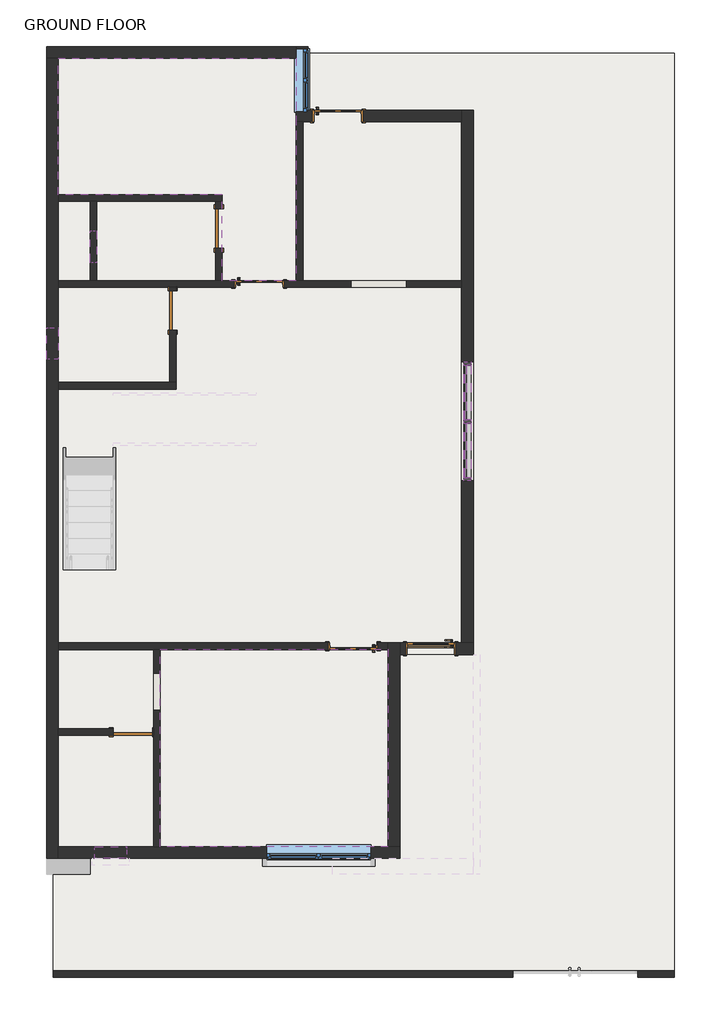
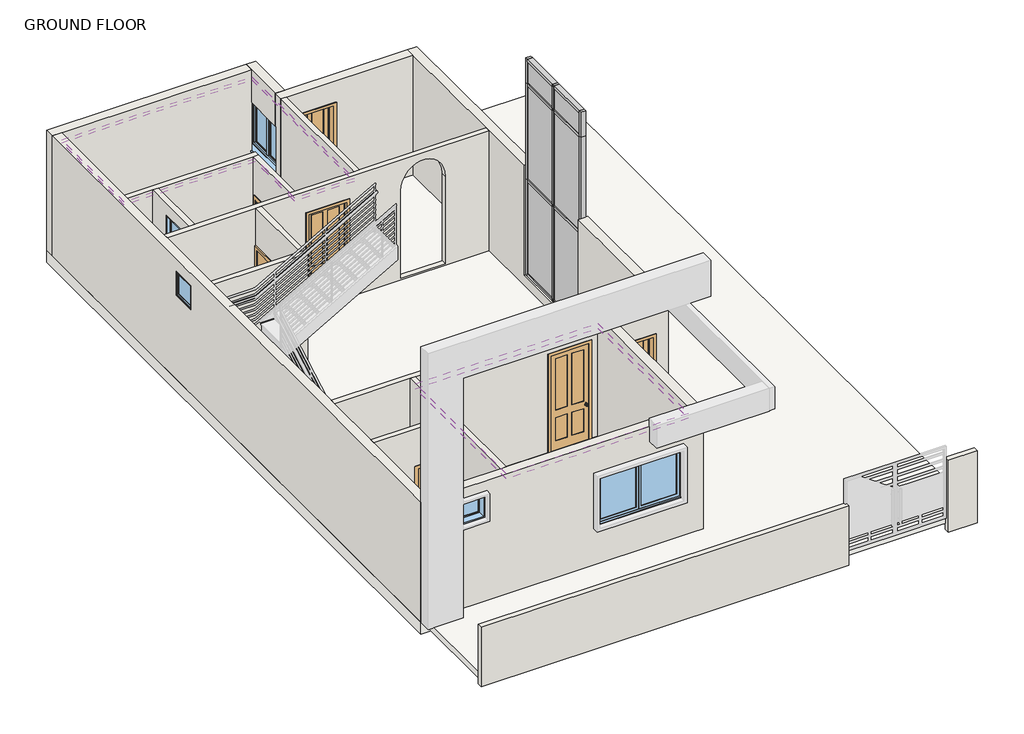
# One storey, part 1 of 3: 20 walls, 17 members, 7 doors, 6 plates, 5 windows, 4 coverings, 3 slabs.
"""IFC4 building model written with IfcOpenShell, lengths in millimetres."""

from ifc_helpers import new_model, si_unit, point, frame, origin, origin_with_axes, place, context, project, spatial, polyline, ellipse_curve, trimmed, outline, extrude, faceted_brep, transform, mapped, element, save
from ifc_brep_helpers import plane_surface, extruded_surface, advanced_brep
from components import door_16625766, door_72f69035, door_4f3f9908, door_1fe7f57d, member_78934672, member_697f972d, member_f0fea5a5, member_ee409385, member_057e2f1d, member_06d1cbbd, system_panel_glazed_cc935e45, system_panel_glazed_66ef8e2c, system_panel_glazed_3447b65c, window_80340324, window_d757e824, w2_window_4_x_4_9dec5fc7, w2_window_6_x_4_7b90d420

model = new_model("IFC4")

# Units and contexts
model_context = context("Model", 3, world=origin())
ifc_project = project(units=[si_unit("LENGTHUNIT", "METRE", prefix="MILLI")], contexts=[model_context])

# Site, building, storey
site = spatial("IfcSite", under=ifc_project)
building = spatial("IfcBuilding", under=site)
storey = spatial("IfcBuildingStorey", under=building, Name="GROUND FLOOR", Elevation=304.8)

# Coverings
placement = place(None, origin())
element("IfcCovering", 1, at=placement, inside=storey, context=model_context, shape_type="SweptSolid", body=[
    extrude(outline(polyline([(-7080.273248, 8978.3133697), (-7080.273248, 11594.5133697), (-2508.273248, 11594.5133697), (-2508.273248, 7327.3133697), (-3930.673248, 7327.3133697), (-3930.673248, 8978.3133697), (-7080.273248, 8978.3133697)]), holes=[polyline([(-6775.473248, 11289.7133697), (-6775.473248, 9283.1133697), (-3625.873248, 9283.1133697), (-3625.873248, 7632.1133697), (-2813.073248, 7632.1133697), (-2813.073248, 11289.7133697), (-6775.473248, 11289.7133697)])]), frame((0.0, 0.0, 3098.8), z_axis=(0.0, 0.0, 1.0), x_axis=(1.0, 0.0, 0.0)), (0.0, 0.0, 1.0), 107.95),
    extrude(outline(polyline([(-3422.673248, 10680.1133697), (-3422.673248, 9892.7133697), (-6165.873248, 9892.7133697), (-6165.873248, 10680.1133697), (-3422.673248, 10680.1133697)])), frame((0.0, 0.0, 3098.8), z_axis=(0.0, 0.0, 1.0), x_axis=(1.0, 0.0, 0.0)), (0.0, 0.0, 1.0), 107.95),
])
element("IfcCovering", 2, ObjectType="METAL STUD WHITE CEILING", at=placement, inside=storey, context=model_context, shape_type="SweptSolid", body=[
    extrude(outline(polyline([(-742.973248, 240.7133697), (-742.973248, -3543.8866303), (-5124.473248, -3543.8866303), (-5124.473248, 240.7133697), (-742.973248, 240.7133697)])), frame((0.0, 0.0, 3175.0), z_axis=(0.0, 0.0, 1.0), x_axis=(1.0, 0.0, 0.0)), (0.0, 0.0, 1.0), 107.95),
])
element("IfcCovering", 3, ObjectType="METAL STUD WHITE CEILING", at=placement, inside=storey, context=model_context, shape_type="SweptSolid", body=[
    extrude(outline(polyline([(-742.973248, 240.7133697), (-742.973248, -3543.8866303), (-5124.473248, -3543.8866303), (-5124.473248, 240.7133697), (-742.973248, 240.7133697)]), holes=[polyline([(-1047.773248, -64.0866303), (-4819.673248, -64.0866303), (-4819.673248, -3239.0866303), (-1047.773248, -3239.0866303), (-1047.773248, -64.0866303)])]), frame((0.0, 0.0, 3048.0), z_axis=(0.0, 0.0, 1.0), x_axis=(1.0, 0.0, 0.0)), (0.0, 0.0, 1.0), 107.95),
])
element("IfcCovering", 4, ObjectType="METAL STUD WHITE CEILING", at=placement, inside=storey, context=model_context, shape_type="SweptSolid", body=[
    extrude(outline(polyline([(-3930.673248, 8978.3133697), (-7080.273248, 8978.3133697), (-7080.273248, 11594.5133697), (-2508.273248, 11594.5133697), (-2508.273248, 10489.6133697), (-2508.273248, 7327.3133697), (-3930.673248, 7327.3133697), (-3930.673248, 8978.3133697)])), frame((0.0, 0.0, 3175.0), z_axis=(0.0, 0.0, 1.0), x_axis=(1.0, 0.0, 0.0)), (0.0, 0.0, 1.0), 107.95),
])

# Doors
door_shape = door_16625766(model_context)
element("IfcDoor", 5, ObjectType="36\" x 84\"", at=placement, inside=storey, context=model_context, shape_type="MappedRepresentation", body=[
    mapped(door_shape, transform((76.176752, 256.5883697, 304.8), x_axis=(1.0, 0.0, 0.0), y_axis=(0.0, 1.0, 0.0), z_axis=(0.0, 0.0, 1.0))),
])
door_2_shape = door_72f69035(model_context)
element("IfcDoor", 6, ObjectType="Door-Interior-Single-4_Panel-Wood : 36\" x 96\"", at=placement, inside=storey, context=model_context, shape_type="MappedRepresentation", body=[
    mapped(door_2_shape, transform((-1416.073248, 301.0383697, 304.8), x_axis=(-1.0, 0.0, 0.0), y_axis=(0.0, -1.0, 0.0), z_axis=(0.0, 0.0, 1.0))),
])
element("IfcDoor", 7, ObjectType="Door-Interior-Single-4_Panel-Wood : 36\" x 96\"", at=placement, inside=storey, context=model_context, shape_type="MappedRepresentation", body=[
    mapped(door_2_shape, transform((-3219.473248, 7266.9883697, 304.8), x_axis=(1.0, 0.0, 0.0), y_axis=(0.0, 1.0, 0.0), z_axis=(0.0, 0.0, 1.0))),
])
door_3_shape = door_4f3f9908(model_context)
element("IfcDoor", 8, ObjectType="Door-Interior-Single-4_Panel-Wood : 36\" x 96\"", at=placement, inside=storey, context=model_context, shape_type="MappedRepresentation", body=[
    mapped(door_3_shape, transform((-1708.173248, 10492.7883697, 304.8), x_axis=(1.0, 0.0, 0.0), y_axis=(0.0, 1.0, 0.0), z_axis=(0.0, 0.0, 1.0))),
])
door_4_shape = door_1fe7f57d(model_context)
element("IfcDoor", 9, ObjectType="Single-Flush : 30\" x 80\"", at=placement, inside=storey, context=model_context, shape_type="MappedRepresentation", body=[
    mapped(door_4_shape, transform((-4883.173248, 6755.8133697, 304.8), x_axis=(0.0, 1.0, 0.0), y_axis=(-1.0, 0.0, 0.0), z_axis=(0.0, 0.0, 1.0))),
])
element("IfcDoor", 10, ObjectType="Single-Flush : 30\" x 80\"", at=placement, inside=storey, context=model_context, shape_type="MappedRepresentation", body=[
    mapped(door_4_shape, transform((-3994.173248, 8330.6133697, 304.8), x_axis=(0.0, 1.0, 0.0), y_axis=(-1.0, 0.0, 0.0), z_axis=(0.0, 0.0, 1.0))),
])
element("IfcDoor", 11, ObjectType="Single-Flush : 30\" x 80\"", at=placement, inside=storey, context=model_context, shape_type="MappedRepresentation", body=[
    mapped(door_4_shape, transform((-5645.173248, -1346.7866303, 304.8), x_axis=(-1.0, 0.0, 0.0), y_axis=(0.0, -1.0, 0.0), z_axis=(0.0, 0.0, 1.0))),
])

# Members
member_shape = member_78934672(model_context)
element("IfcMember", 12, ObjectType="Rectangular Mullion : 2.5\" x 5\" rectangular", at=placement, inside=storey, context=model_context, shape_type="MappedRepresentation", body=[
    mapped(member_shape, transform((781.026752, 5701.7133697, 6059.5090117), x_axis=(0.0, 0.0, 1.0), y_axis=(1.0, 0.0, 0.0), z_axis=(0.0, 1.0, 0.0))),
])
element("IfcMember", 13, ObjectType="Rectangular Mullion : 2.5\" x 5\" rectangular", at=placement, inside=storey, context=model_context, shape_type="MappedRepresentation", body=[
    mapped(member_shape, transform((781.026752, 4590.4633697, 6059.5090117), x_axis=(0.0, 0.0, 1.0), y_axis=(1.0, 0.0, 0.0), z_axis=(0.0, 1.0, 0.0))),
])
element("IfcMember", 14, ObjectType="Rectangular Mullion : 2.5\" x 5\" rectangular", at=placement, inside=storey, context=model_context, shape_type="MappedRepresentation", body=[
    mapped(member_shape, transform((781.026752, 3542.7133697, 546.4883491), x_axis=(0.0, 0.0, -1.0), y_axis=(1.0, 0.0, 0.0), z_axis=(0.0, -1.0, 0.0))),
])
element("IfcMember", 15, ObjectType="Rectangular Mullion : 2.5\" x 5\" rectangular", at=placement, inside=storey, context=model_context, shape_type="MappedRepresentation", body=[
    mapped(member_shape, transform((781.026752, 4653.9633697, 546.4883491), x_axis=(0.0, 0.0, -1.0), y_axis=(1.0, 0.0, 0.0), z_axis=(0.0, -1.0, 0.0))),
])
member_2_shape = member_697f972d(model_context)
element("IfcMember", 16, ObjectType="Rectangular Mullion : 2.5\" x 5\" rectangular", at=placement, inside=storey, context=model_context, shape_type="MappedRepresentation", body=[
    mapped(member_2_shape, transform((781.026752, 4590.4633697, 2984.8883491), x_axis=(0.0, 0.0, 1.0), y_axis=(1.0, 0.0, 0.0), z_axis=(0.0, 1.0, 0.0))),
])
element("IfcMember", 17, ObjectType="Rectangular Mullion : 2.5\" x 5\" rectangular", at=placement, inside=storey, context=model_context, shape_type="MappedRepresentation", body=[
    mapped(member_2_shape, transform((781.026752, 5701.7133697, 2984.8883491), x_axis=(0.0, 0.0, 1.0), y_axis=(1.0, 0.0, 0.0), z_axis=(0.0, 1.0, 0.0))),
])
element("IfcMember", 18, ObjectType="Rectangular Mullion : 2.5\" x 5\" rectangular", at=placement, inside=storey, context=model_context, shape_type="MappedRepresentation", body=[
    mapped(member_2_shape, transform((781.026752, 4590.4633697, 5423.2883491), x_axis=(0.0, 0.0, 1.0), y_axis=(1.0, 0.0, 0.0), z_axis=(0.0, 1.0, 0.0))),
])
element("IfcMember", 19, ObjectType="Rectangular Mullion : 2.5\" x 5\" rectangular", at=placement, inside=storey, context=model_context, shape_type="MappedRepresentation", body=[
    mapped(member_2_shape, transform((781.026752, 5701.7133697, 5423.2883491), x_axis=(0.0, 0.0, 1.0), y_axis=(1.0, 0.0, 0.0), z_axis=(0.0, 1.0, 0.0))),
])
member_3_shape = member_f0fea5a5(model_context)
element("IfcMember", 20, ObjectType="Rectangular Mullion : 2.5\" x 5\" rectangular", at=placement, inside=storey, context=model_context, shape_type="MappedRepresentation", body=[
    mapped(member_3_shape, transform((781.026752, 4622.2133697, 546.4883491), x_axis=(0.0, 1.0, 0.0), y_axis=(1.0, 0.0, 0.0), z_axis=(0.0, 0.0, -1.0))),
])
member_4_shape = member_ee409385(model_context)
element("IfcMember", 21, ObjectType="Rectangular Mullion : 2.5\" x 5\" rectangular", at=placement, inside=storey, context=model_context, shape_type="MappedRepresentation", body=[
    mapped(member_4_shape, transform((781.026752, 5765.2133697, 546.4883491), x_axis=(0.0, 1.0, 0.0), y_axis=(1.0, 0.0, 0.0), z_axis=(0.0, 0.0, -1.0))),
])
element("IfcMember", 22, ObjectType="Rectangular Mullion : 2.5\" x 5\" rectangular", at=placement, inside=storey, context=model_context, shape_type="MappedRepresentation", body=[
    mapped(member_4_shape, transform((781.026752, 3479.2133697, 2984.8883491), x_axis=(0.0, -1.0, 0.0), y_axis=(1.0, 0.0, 0.0), z_axis=(0.0, 0.0, 1.0))),
])
element("IfcMember", 23, ObjectType="Rectangular Mullion : 2.5\" x 5\" rectangular", at=placement, inside=storey, context=model_context, shape_type="MappedRepresentation", body=[
    mapped(member_3_shape, transform((781.026752, 4622.2133697, 2984.8883491), x_axis=(0.0, 1.0, 0.0), y_axis=(1.0, 0.0, 0.0), z_axis=(0.0, 0.0, -1.0))),
])
element("IfcMember", 24, ObjectType="Rectangular Mullion : 2.5\" x 5\" rectangular", at=placement, inside=storey, context=model_context, shape_type="MappedRepresentation", body=[
    mapped(member_4_shape, transform((781.026752, 5765.2133697, 2984.8883491), x_axis=(0.0, 1.0, 0.0), y_axis=(1.0, 0.0, 0.0), z_axis=(0.0, 0.0, -1.0))),
])
element("IfcMember", 25, ObjectType="Rectangular Mullion : 2.5\" x 5\" rectangular", at=placement, inside=storey, context=model_context, shape_type="MappedRepresentation", body=[
    mapped(member_4_shape, transform((781.026752, 3479.2133697, 5423.2883491), x_axis=(0.0, -1.0, 0.0), y_axis=(1.0, 0.0, 0.0), z_axis=(0.0, 0.0, 1.0))),
])
member_5_shape = member_057e2f1d(model_context)
element("IfcMember", 26, ObjectType="Rectangular Mullion : 2.5\" x 5\" rectangular", at=placement, inside=storey, context=model_context, shape_type="MappedRepresentation", body=[
    mapped(member_5_shape, transform((781.026752, 4622.2133697, 5423.2883491), x_axis=(0.0, 1.0, 0.0), y_axis=(1.0, 0.0, 0.0), z_axis=(0.0, 0.0, -1.0))),
])
member_6_shape = member_06d1cbbd(model_context)
element("IfcMember", 27, ObjectType="Rectangular Mullion : 2.5\" x 5\" rectangular", at=placement, inside=storey, context=model_context, shape_type="MappedRepresentation", body=[
    mapped(member_6_shape, transform((781.026752, 3479.2133697, 6059.5090117), x_axis=(0.0, -1.0, 0.0), y_axis=(1.0, 0.0, 0.0), z_axis=(0.0, 0.0, 1.0))),
])
element("IfcMember", 28, ObjectType="Rectangular Mullion : 2.5\" x 5\" rectangular", at=placement, inside=storey, context=model_context, shape_type="MappedRepresentation", body=[
    mapped(member_6_shape, transform((781.026752, 5765.2133697, 5423.2883491), x_axis=(0.0, 1.0, 0.0), y_axis=(1.0, 0.0, 0.0), z_axis=(0.0, 0.0, -1.0))),
])

# Plates
system_panel_glazed_shape = system_panel_glazed_cc935e45(model_context)
element("IfcPlate", 29, ObjectType="System Panel : Glazed", at=placement, inside=storey, context=model_context, shape_type="MappedRepresentation", body=[
    mapped(system_panel_glazed_shape, transform((781.026752, 4066.5883697, 609.9883491), x_axis=(0.0, 1.0, 0.0), y_axis=(-1.0, 0.0, 0.0), z_axis=(0.0, 0.0, 1.0))),
])
element("IfcPlate", 30, ObjectType="System Panel : Glazed", at=placement, inside=storey, context=model_context, shape_type="MappedRepresentation", body=[
    mapped(system_panel_glazed_shape, transform((781.026752, 5177.8383697, 609.9883491), x_axis=(0.0, 1.0, 0.0), y_axis=(-1.0, 0.0, 0.0), z_axis=(0.0, 0.0, 1.0))),
])
system_panel_glazed_2_shape = system_panel_glazed_66ef8e2c(model_context)
element("IfcPlate", 31, ObjectType="System Panel : Glazed", at=placement, inside=storey, context=model_context, shape_type="MappedRepresentation", body=[
    mapped(system_panel_glazed_2_shape, transform((781.026752, 4066.5883697, 3016.6383491), x_axis=(0.0, 1.0, 0.0), y_axis=(-1.0, 0.0, 0.0), z_axis=(0.0, 0.0, 1.0))),
])
element("IfcPlate", 32, ObjectType="System Panel : Glazed", at=placement, inside=storey, context=model_context, shape_type="MappedRepresentation", body=[
    mapped(system_panel_glazed_2_shape, transform((781.026752, 5177.8383697, 3016.6383491), x_axis=(0.0, 1.0, 0.0), y_axis=(-1.0, 0.0, 0.0), z_axis=(0.0, 0.0, 1.0))),
])
system_panel_glazed_3_shape = system_panel_glazed_3447b65c(model_context)
element("IfcPlate", 33, ObjectType="System Panel : Glazed", at=placement, inside=storey, context=model_context, shape_type="MappedRepresentation", body=[
    mapped(system_panel_glazed_3_shape, transform((781.026752, 4066.5883697, 5455.0383491), x_axis=(0.0, 1.0, 0.0), y_axis=(-1.0, 0.0, 0.0), z_axis=(0.0, 0.0, 1.0))),
])
element("IfcPlate", 34, ObjectType="System Panel : Glazed", at=placement, inside=storey, context=model_context, shape_type="MappedRepresentation", body=[
    mapped(system_panel_glazed_3_shape, transform((781.026752, 5177.8383697, 5455.0383491), x_axis=(0.0, 1.0, 0.0), y_axis=(-1.0, 0.0, 0.0), z_axis=(0.0, 0.0, 1.0))),
])

# Slabs
element("IfcSlab", 35, at=placement, inside=storey, context=model_context, shape_type="SweptSolid", body=[
    extrude(outline(polyline([(-5251.473248, -3543.8866303), (-7080.273248, -3543.8866303), (-7080.273248, -1410.2866303), (-5251.473248, -1410.2866303), (-5251.473248, -3543.8866303)])), origin_with_axes(), (0.0, 0.0, 1.0), 304.8),
    extrude(outline(polyline([(-4946.673248, 7200.3133697), (-4946.673248, 5371.5133697), (-7080.273248, 5371.5133697), (-7080.273248, 7200.3133697), (-4946.673248, 7200.3133697)])), origin_with_axes(), (0.0, 0.0, 1.0), 304.8),
    extrude(outline(polyline([(-4057.673248, 8851.3133697), (-4057.673248, 7327.3133697), (-6343.673248, 7327.3133697), (-6343.673248, 8851.3133697), (-4057.673248, 8851.3133697)])), origin_with_axes(), (0.0, 0.0, 1.0), 304.8),
])
element("IfcSlab", 36, at=placement, inside=storey, context=model_context, shape_type="SweptSolid", body=[
    extrude(outline(polyline([(-514.373248, -3772.4866303), (-514.373248, 139.1133697), (895.326752, 139.1133697), (895.326752, 10603.9133697), (-2279.673248, 10603.9133697), (-2279.673248, 11696.1133697), (4756.126752, 11696.1133697), (4756.126752, -5931.4866303), (-7181.873248, -5931.4866303), (-7181.873248, -3772.4866303), (-514.373248, -3772.4866303)])), frame((0.0, 0.0, 152.4), z_axis=(0.0, 0.0, 1.0), x_axis=(1.0, 0.0, 0.0)), (0.0, 0.0, 1.0), 152.4),
])
element("IfcSlab", 37, ObjectType="MARBLE FLOORING 1'", at=placement, inside=storey, context=model_context, shape_type="SweptSolid", body=[
    extrude(outline(polyline([(-514.373248, -3772.4866303), (-7308.873248, -3772.4866303), (-7308.873248, 11823.1133697), (-2279.673248, 11823.1133697), (-2279.673248, 10603.9133697), (895.326752, 10603.9133697), (895.326752, 139.1133697), (-514.373248, 139.1133697), (-514.373248, -3772.4866303)]), holes=[polyline([(-4057.673248, 8851.3133697), (-6343.673248, 8851.3133697), (-6343.673248, 7327.3133697), (-4057.673248, 7327.3133697), (-4057.673248, 8851.3133697)]), polyline([(-4946.673248, 7200.3133697), (-7080.273248, 7200.3133697), (-7080.273248, 5371.5133697), (-4946.673248, 5371.5133697), (-4946.673248, 7200.3133697)]), polyline([(-5251.473248, -3543.8866303), (-5251.473248, -1410.2866303), (-7080.273248, -1410.2866303), (-7080.273248, -3543.8866303), (-5251.473248, -3543.8866303)])]), origin_with_axes(), (0.0, 0.0, 1.0), 304.8),
])

# Walls
element("IfcWall", 38, ObjectType="INNER WALL 5\"", at=placement, inside=storey, context=model_context, shape_type="AdvancedBrep", body=[
    advanced_brep(
    [(-5124.473248, -3543.8866303, 304.8), (-5124.473248, 240.7133697, 304.8), (-5124.473248, 240.7133697, 3352.8), (-5124.473248, -3543.8866303, 3352.8), (-5124.473248, -211.107669, 445.0989834), (-5124.473248, -921.3329942, 445.0989834), (-5124.473248, -921.3329942, 2667.1596494), (-5124.473248, -211.107669, 2629.9383173), (-5251.473248, -3543.8866303, 304.8), (-5251.473248, -3543.8866303, 3352.8), (-5251.473248, -1410.2866303, 3352.8), (-5251.473248, -1283.2866303, 3352.8), (-5251.473248, 240.7133697, 3352.8), (-5251.473248, 240.7133697, 304.8), (-5251.473248, -1283.2866303, 304.8), (-5251.473248, -1410.2866303, 304.8), (-5251.473248, -211.107669, 445.0989834), (-5251.473248, -211.107669, 2629.9383173), (-5251.473248, -921.3329942, 2667.1596494), (-5251.473248, -921.3329942, 445.0989834)],
    [
        (0, 1),
        (1, 2),
        (2, 3),
        (3, 0),
        (4, 5),
        (5, 6),
        (6, 7, ellipse_curve(frame((-5124.473248, -566.2203316, 2648.5489834), z_axis=(-1.0, 0.0, 0.0), x_axis=(0.0, -0.052335956242941746, -0.998629534754574)), 457.2, 355.6)),
        (7, 4),
        (8, 9),
        (9, 10),
        (10, 11),
        (11, 12),
        (12, 13),
        (13, 14),
        (14, 15),
        (15, 8),
        (16, 17),
        (17, 18, ellipse_curve(frame((-5251.473248, -566.2203316, 2648.5489834), z_axis=(1.0, 0.0, 0.0), x_axis=(0.0, -0.052335956242941746, -0.998629534754574)), 457.2, 355.6)),
        (18, 19),
        (19, 16),
        (3, 9),
        (8, 0),
        (1, 13),
        (12, 2),
        (4, 16),
        (19, 5),
        (18, 6),
        (17, 7),
    ],
    [
        plane_surface(frame((-5124.473248, -3543.8866303, 304.8), z_axis=(1.0, 0.0, 0.0), x_axis=(0.0, 1.0, 0.0))),
        plane_surface(frame((-5251.473248, -3543.8866303, 304.8), z_axis=(-1.0, 0.0, 0.0), x_axis=(0.0, -1.0, 0.0))),
        plane_surface(frame((-7219.973248, -3543.8866303, 304.8), z_axis=(0.0, -1.0, 0.0), x_axis=(-1.0, 0.0, 0.0))),
        plane_surface(frame((-742.973248, 240.7133697, 304.8), z_axis=(0.0, 1.0, 0.0), x_axis=(1.0, 0.0, 0.0))),
        plane_surface(frame((-5124.473248, -3658.1866303, 304.8), z_axis=(0.0, 0.0, -1.0), x_axis=(-1.0, 0.0, 0.0))),
        plane_surface(frame((-5124.473248, 304.2133697, 3352.8), z_axis=(0.0, 0.0, 1.0), x_axis=(-1.0, 0.0, 0.0))),
        plane_surface(frame((-5124.473248, -211.107669, 445.0989834), z_axis=(0.0, 0.0, 1.0), x_axis=(-1.0, 0.0, 0.0))),
        plane_surface(frame((-5124.473248, -921.3329942, 445.0989834), z_axis=(0.0, 1.0, 0.0), x_axis=(-1.0, 0.0, 0.0))),
        extruded_surface(trimmed(ellipse_curve(frame((-5314.973248, -566.2203316, 2648.5489834), z_axis=(-1.0, 0.0, 0.0), x_axis=(0.0, 0.998629534754574, -0.052335956242941746)), 355.6, 457.2), [point((-5314.973248, -921.3329942, 2667.1596494))], [point((-5314.973248, -211.107669, 2629.9383173))], True, "CARTESIAN"), (127.0, 0.0, 0.0), 127.0),
        plane_surface(frame((-5124.473248, -211.107669, 2629.9383173), z_axis=(0.0, -1.0, 0.0), x_axis=(-1.0, 0.0, 0.0))),
    ],
    [
        (0, [[1, 2, 3, 4], [5, 6, 7, 8]]),
        (1, [[9, 10, 11, 12, 13, 14, 15, 16], [17, 18, 19, 20]]),
        (2, [[-4, 21, -9, 22]]),
        (3, [[-2, 23, -13, 24]]),
        (4, [[-1, -22, -16, -15, -14, -23]]),
        (5, [[-3, -24, -12, -11, -10, -21]]),
        (6, [[-5, 25, -20, 26]]),
        (7, [[-6, -26, -19, 27]]),
        (8, [[-7, -27, -18, 28]]),
        (9, [[-8, -28, -17, -25]]),
    ],
),
])
element("IfcWall", 39, ObjectType="INNER WALL 5\"", at=placement, inside=storey, context=model_context, shape_type="SweptSolid", body=[
    extrude(outline(polyline([(304.8, -7080.273248), (304.8, -6026.173248), (2336.8, -6026.173248), (2336.8, -5264.173248), (304.8, -5264.173248), (304.8, -5251.473248), (3352.8, -5251.473248), (3352.8, -7080.273248), (304.8, -7080.273248)])), frame((0.0, -1410.2866303, 0.0), z_axis=(0.0, 1.0, 0.0), x_axis=(0.0, 0.0, 1.0)), (0.0, 0.0, 1.0), 127.0),
])
element("IfcWall", 40, ObjectType="INNER WALL 5\"", at=placement, inside=storey, context=model_context, shape_type="Brep", body=[
    faceted_brep([(-7080.273248, 367.7133697, 3352.8), (-742.973248, 367.7133697, 3352.8), (-742.973248, 367.7133697, 304.8), (-933.473248, 367.7133697, 304.8), (-933.473248, 367.7133697, 2768.6), (-1898.673248, 367.7133697, 2768.6), (-1898.673248, 367.7133697, 304.8), (-7080.273248, 367.7133697, 304.8), (-742.973248, 240.7133697, 3352.8), (-5124.473248, 240.7133697, 3352.8), (-5251.473248, 240.7133697, 3352.8), (-7080.273248, 240.7133697, 3352.8), (-7080.273248, 240.7133697, 304.8), (-5251.473248, 240.7133697, 304.8), (-5124.473248, 240.7133697, 304.8), (-1898.673248, 240.7133697, 304.8), (-1898.673248, 240.7133697, 2768.6), (-933.473248, 240.7133697, 2768.6), (-933.473248, 240.7133697, 304.8), (-742.973248, 240.7133697, 304.8)], [[[0, 1, 2, 3, 4, 5, 6, 7]], [[8, 9, 10, 11, 12, 13, 14, 15, 16, 17, 18, 19]], [[2, 19, 18, 3]], [[12, 7, 6, 15, 14, 13]], [[1, 0, 11, 10, 9, 8]], [[2, 1, 8, 19]], [[0, 7, 12, 11]], [[5, 16, 15, 6]], [[16, 5, 4, 17]], [[17, 4, 3, 18]]]),
])
element("IfcWall", 41, ObjectType="INNER WALL 5\"", at=placement, inside=storey, context=model_context, shape_type="AdvancedBrep", body=[
    advanced_brep(
    [(666.726752, 7200.3133697, 3352.8), (-4819.673248, 7200.3133697, 3352.8), (-4946.673248, 7200.3133697, 3352.8), (-7080.273248, 7200.3133697, 3352.8), (-7080.273248, 7200.3133697, 304.8), (-4946.673248, 7200.3133697, 304.8), (-4819.673248, 7200.3133697, 304.8), (-3702.073248, 7200.3133697, 304.8), (-3702.073248, 7200.3133697, 2768.6), (-2736.873248, 7200.3133697, 2768.6), (-2736.873248, 7200.3133697, 304.8), (666.726752, 7200.3133697, 304.8), (-387.8615631, 7200.3133697, 344.0138877), (-1454.6615631, 7200.3133697, 344.0138877), (-1454.6615631, 7200.3133697, 2318.5977751), (-1454.6615631, 7200.3133697, 2566.5138877), (-387.8615631, 7200.3133697, 2566.5138877), (-7080.273248, 7327.3133697, 3352.8), (-6470.673248, 7327.3133697, 3352.8), (-6343.673248, 7327.3133697, 3352.8), (-4057.673248, 7327.3133697, 3352.8), (-3930.673248, 7327.3133697, 3352.8), (-2508.273248, 7327.3133697, 3352.8), (-2381.273248, 7327.3133697, 3352.8), (666.726752, 7327.3133697, 3352.8), (666.726752, 7327.3133697, 304.8), (-2381.273248, 7327.3133697, 304.8), (-2508.273248, 7327.3133697, 304.8), (-2736.873248, 7327.3133697, 304.8), (-2736.873248, 7327.3133697, 2768.6), (-3702.073248, 7327.3133697, 2768.6), (-3702.073248, 7327.3133697, 304.8), (-3930.673248, 7327.3133697, 304.8), (-4057.673248, 7327.3133697, 304.8), (-6343.673248, 7327.3133697, 304.8), (-6470.673248, 7327.3133697, 304.8), (-7080.273248, 7327.3133697, 304.8), (-1454.6615631, 7327.3133697, 344.0138877), (-387.8615631, 7327.3133697, 344.0138877), (-387.8615631, 7327.3133697, 2566.5138877), (-1454.6615631, 7327.3133697, 2566.5138877), (-1454.6615631, 7327.3133697, 2318.5977751)],
    [
        (0, 1),
        (1, 2),
        (2, 3),
        (3, 4),
        (4, 5),
        (5, 6),
        (6, 7),
        (7, 8),
        (8, 9),
        (9, 10),
        (10, 11),
        (11, 0),
        (12, 13),
        (13, 14),
        (14, 15),
        (15, 16, ellipse_curve(frame((-921.2615631, 7200.3133697, 2566.5138877), z_axis=(0.0, 1.0, 0.0), x_axis=(0.0, 0.0, -1.0)), 609.6, 533.4)),
        (16, 12),
        (17, 18),
        (18, 19),
        (19, 20),
        (20, 21),
        (21, 22),
        (22, 23),
        (23, 24),
        (24, 25),
        (25, 26),
        (26, 27),
        (27, 28),
        (28, 29),
        (29, 30),
        (30, 31),
        (31, 32),
        (32, 33),
        (33, 34),
        (34, 35),
        (35, 36),
        (36, 17),
        (37, 38),
        (38, 39),
        (39, 40, ellipse_curve(frame((-921.2615631, 7327.3133697, 2566.5138877), z_axis=(0.0, -1.0, 0.0), x_axis=(0.0, 0.0, -1.0)), 609.6, 533.4)),
        (40, 41),
        (41, 37),
        (3, 17),
        (36, 4),
        (11, 25),
        (24, 0),
        (31, 7),
        (10, 28),
        (12, 38),
        (37, 13),
        (41, 14),
        (40, 15),
        (39, 16),
        (9, 29),
        (8, 30),
    ],
    [
        plane_surface(frame((-6991.373248, 7200.3133697, 304.8), z_axis=(0.0, -1.0, 0.0), x_axis=(1.0, 0.0, 0.0))),
        plane_surface(frame((-6991.373248, 7327.3133697, 304.8), z_axis=(0.0, 1.0, 0.0), x_axis=(-1.0, 0.0, 0.0))),
        plane_surface(frame((-7080.273248, 8571.9133697, 304.8), z_axis=(-1.0, 0.0, 0.0), x_axis=(0.0, 1.0, 0.0))),
        plane_surface(frame((666.726752, 1256.7133697, 304.8), z_axis=(1.0, 0.0, 0.0), x_axis=(0.0, -1.0, 0.0))),
        plane_surface(frame((-7194.573248, 7200.3133697, 304.8), z_axis=(0.0, 0.0, -1.0), x_axis=(0.0, 1.0, 0.0))),
        plane_surface(frame((781.026752, 7200.3133697, 3352.8), z_axis=(0.0, 0.0, 1.0), x_axis=(0.0, 1.0, 0.0))),
        plane_surface(frame((-387.8615631, 7200.3133697, 344.0138877), z_axis=(0.0, 0.0, 1.0), x_axis=(0.0, 1.0, 0.0))),
        plane_surface(frame((-1454.6615631, 7200.3133697, 344.0138877), z_axis=(1.0, 0.0, 0.0), x_axis=(0.0, 1.0, 0.0))),
        plane_surface(frame((-1454.6615631, 7200.3133697, 2318.5977751), z_axis=(1.0, 0.0, 0.0), x_axis=(0.0, 1.0, 0.0))),
        extruded_surface(trimmed(ellipse_curve(frame((-921.2615631, 7390.8133697, 2566.5138877), z_axis=(0.0, 1.0, 0.0), x_axis=(1.0, 0.0, 0.0)), 533.4, 609.6), [point((-1454.6615631, 7390.8133697, 2566.5138877))], [point((-387.8615631, 7390.8133697, 2566.5138877))], True, "CARTESIAN"), (0.0, -127.0, 0.0), 127.0),
        plane_surface(frame((-387.8615631, 7200.3133697, 2566.5138877), z_axis=(-1.0, 0.0, 0.0), x_axis=(0.0, 1.0, 0.0))),
        plane_surface(frame((-2736.873248, 5676.3133697, 304.8), z_axis=(-1.0, 0.0, 0.0), x_axis=(0.0, 1.0, 0.0))),
        plane_surface(frame((-2736.873248, 5676.3133697, 2768.6), z_axis=(0.0, 0.0, -1.0), x_axis=(0.0, 1.0, 0.0))),
        plane_surface(frame((-3702.073248, 5676.3133697, 2768.6), z_axis=(1.0, 0.0, 0.0), x_axis=(0.0, 1.0, 0.0))),
    ],
    [
        (0, [[1, 2, 3, 4, 5, 6, 7, 8, 9, 10, 11, 12], [13, 14, 15, 16, 17]]),
        (1, [[18, 19, 20, 21, 22, 23, 24, 25, 26, 27, 28, 29, 30, 31, 32, 33, 34, 35, 36, 37], [38, 39, 40, 41, 42]]),
        (2, [[-4, 43, -37, 44]]),
        (3, [[-12, 45, -25, 46]]),
        (4, [[-44, -36, -35, -34, -33, -32, 47, -7, -6, -5]]),
        (4, [[-45, -11, 48, -28, -27, -26]]),
        (5, [[-3, -2, -1, -46, -24, -23, -22, -21, -20, -19, -18, -43]]),
        (6, [[-13, 49, -38, 50]]),
        (7, [[-14, -50, -42, 51]]),
        (8, [[-15, -51, -41, 52]]),
        (9, [[-16, -52, -40, 53]]),
        (10, [[-17, -53, -39, -49]]),
        (11, [[54, -29, -48, -10]]),
        (12, [[-54, -9, 55, -30]]),
        (13, [[-55, -8, -47, -31]]),
    ],
),
])
element("IfcWall", 42, ObjectType="INNER WALL 5\"", at=placement, inside=storey, context=model_context, shape_type="SweptSolid", body=[
    extrude(outline(polyline([(-2508.273248, 7327.3133697), (-2508.273248, 10375.3133697), (-2381.273248, 10375.3133697), (-2381.273248, 7327.3133697), (-2508.273248, 7327.3133697)])), frame((0.0, 0.0, 304.8), z_axis=(0.0, 0.0, 1.0), x_axis=(1.0, 0.0, 0.0)), (0.0, 0.0, 1.0), 3048.0),
])
element("IfcWall", 43, ObjectType="INNER WALL 5\"", at=placement, inside=storey, context=model_context, shape_type="Brep", body=[
    faceted_brep([(-7080.273248, 5244.5133697, 304.8), (-4819.673248, 5244.5133697, 304.8), (-4819.673248, 5244.5133697, 3352.8), (-7080.273248, 5244.5133697, 3352.8), (-7080.273248, 5371.5133697, 304.8), (-7080.273248, 5371.5133697, 3352.8), (-4946.673248, 5371.5133697, 3352.8), (-4819.673248, 5371.5133697, 3352.8), (-4819.673248, 5371.5133697, 304.8), (-4946.673248, 5371.5133697, 304.8)], [[[0, 1, 2, 3]], [[4, 5, 6, 7, 8, 9]], [[1, 0, 4, 9, 8]], [[3, 2, 7, 6, 5]], [[0, 3, 5, 4]], [[2, 1, 8, 7]]]),
])
element("IfcWall", 44, ObjectType="INNER WALL 5\"", at=placement, inside=storey, context=model_context, shape_type="SweptSolid", body=[
    extrude(outline(polyline([(7200.3133697, 304.8), (7136.8133697, 304.8), (7136.8133697, 2336.8), (6374.8133697, 2336.8), (6374.8133697, 304.8), (5371.5133697, 304.8), (5371.5133697, 3352.8), (7200.3133697, 3352.8), (7200.3133697, 304.8)])), frame((-4946.673248, 0.0, 0.0), z_axis=(1.0, 0.0, 0.0), x_axis=(0.0, 1.0, 0.0)), (0.0, 0.0, 1.0), 127.0),
])
element("IfcWall", 45, ObjectType="INNER WALL 5\"", at=placement, inside=storey, context=model_context, shape_type="Brep", body=[
    faceted_brep([(-7080.273248, 8851.3133697, 304.8), (-6470.673248, 8851.3133697, 304.8), (-6343.673248, 8851.3133697, 304.8), (-4057.673248, 8851.3133697, 304.8), (-3930.673248, 8851.3133697, 304.8), (-3930.673248, 8851.3133697, 3352.8), (-4057.673248, 8851.3133697, 3352.8), (-6343.673248, 8851.3133697, 3352.8), (-6470.673248, 8851.3133697, 3352.8), (-7080.273248, 8851.3133697, 3352.8), (-7080.273248, 8978.3133697, 304.8), (-7080.273248, 8978.3133697, 3352.8), (-3930.673248, 8978.3133697, 3352.8), (-3930.673248, 8978.3133697, 304.8)], [[[0, 1, 2, 3, 4, 5, 6, 7, 8, 9]], [[10, 11, 12, 13]], [[4, 3, 2, 1, 0, 10, 13]], [[9, 8, 7, 6, 5, 12, 11]], [[0, 9, 11, 10]], [[5, 4, 13, 12]]]),
])
element("IfcWall", 46, ObjectType="INNER WALL 5\"", at=placement, inside=storey, context=model_context, shape_type="SweptSolid", body=[
    extrude(outline(polyline([(7327.3133697, 3352.8), (8851.3133697, 3352.8), (8851.3133697, 304.8), (8711.6133697, 304.8), (8711.6133697, 2336.8), (7949.6133697, 2336.8), (7949.6133697, 304.8), (7327.3133697, 304.8), (7327.3133697, 3352.8)])), frame((-4057.673248, 0.0, 0.0), z_axis=(1.0, 0.0, 0.0), x_axis=(0.0, 1.0, 0.0)), (0.0, 0.0, 1.0), 127.0),
])
element("IfcWall", 47, ObjectType="INNER WALL 5\"", at=placement, inside=storey, context=model_context, shape_type="SweptSolid", body=[
    extrude(outline(polyline([(8851.3133697, 304.8), (7327.3133697, 304.8), (7327.3133697, 3352.8), (8851.3133697, 3352.8), (8851.3133697, 304.8)]), holes=[polyline([(7670.2133697, 3048.0), (7670.2133697, 2438.4), (8279.8133697, 2438.4), (8279.8133697, 3048.0), (7670.2133697, 3048.0)])]), frame((-6470.673248, 0.0, 0.0), z_axis=(1.0, 0.0, 0.0), x_axis=(0.0, 1.0, 0.0)), (0.0, 0.0, 1.0), 127.0),
])
element("IfcWall", 48, ObjectType="INNER WALL 5\"", at=placement, inside=storey, context=model_context, shape_type="SweptSolid", body=[
    extrude(outline(polyline([(1657.326752, -6058.4866303), (-7181.873248, -6058.4866303), (-7181.873248, -5931.4866303), (1657.326752, -5931.4866303), (1657.326752, -6058.4866303)])), origin_with_axes(), (0.0, 0.0, 1.0), 1516.6903378),
])
element("IfcWall", 49, ObjectType="INNER WALL 5\"", at=placement, inside=storey, context=model_context, shape_type="Brep", body=[
    faceted_brep([(4756.126752, -5931.4866303, 0.0), (4057.626752, -5931.4866303, 0.0), (4057.626752, -5931.4866303, 1828.8), (4756.126752, -5931.4866303, 1828.8), (4756.126752, -6058.4866303, 0.0), (4756.126752, -6058.4866303, 1524.0), (4756.126752, -6058.4866303, 1828.8), (4057.626752, -6058.4866303, 1828.8), (4057.626752, -6058.4866303, 0.0)], [[[0, 1, 2, 3]], [[4, 5, 6, 7, 8]], [[1, 0, 4, 8]], [[2, 1, 8, 7]], [[3, 2, 7, 6]], [[0, 3, 6, 5, 4]]]),
])
element("IfcWall", 50, ObjectType="OUTER WALL 9\"", at=placement, inside=storey, context=model_context, shape_type="Brep", body=[
    faceted_brep([(-7308.873248, 11594.5133697, 304.8), (-7308.873248, -3772.4866303, 304.8), (-7308.873248, -3772.4866303, 1524.0), (-7308.873248, -3772.4866303, 3352.8), (-7308.873248, 11594.5133697, 3352.8), (-7308.873248, 6425.6133697, 3048.0), (-7308.873248, 5816.0133697, 3048.0), (-7308.873248, 5816.0133697, 2438.4), (-7308.873248, 6425.6133697, 2438.4), (-7080.273248, 11594.5133697, 304.8), (-7080.273248, 11594.5133697, 3352.8), (-7080.273248, 8978.3133697, 3352.8), (-7080.273248, 8851.3133697, 3352.8), (-7080.273248, 7327.3133697, 3352.8), (-7080.273248, 7200.3133697, 3352.8), (-7080.273248, 5371.5133697, 3352.8), (-7080.273248, 5244.5133697, 3352.8), (-7080.273248, 367.7133697, 3352.8), (-7080.273248, 240.7133697, 3352.8), (-7080.273248, -1283.2866303, 3352.8), (-7080.273248, -1410.2866303, 3352.8), (-7080.273248, -3543.8866303, 3352.8), (-7080.273248, -3772.4866303, 3352.8), (-7080.273248, -3772.4866303, 304.8), (-7080.273248, -3543.8866303, 304.8), (-7080.273248, -1410.2866303, 304.8), (-7080.273248, -1283.2866303, 304.8), (-7080.273248, 240.7133697, 304.8), (-7080.273248, 367.7133697, 304.8), (-7080.273248, 5244.5133697, 304.8), (-7080.273248, 5371.5133697, 304.8), (-7080.273248, 7200.3133697, 304.8), (-7080.273248, 7327.3133697, 304.8), (-7080.273248, 8851.3133697, 304.8), (-7080.273248, 8978.3133697, 304.8), (-7080.273248, 6425.6133697, 3048.0), (-7080.273248, 6425.6133697, 2438.4), (-7080.273248, 5816.0133697, 2438.4), (-7080.273248, 5816.0133697, 3048.0)], [[[0, 1, 2, 3, 4], [5, 6, 7, 8]], [[9, 10, 11, 12, 13, 14, 15, 16, 17, 18, 19, 20, 21, 22, 23, 24, 25, 26, 27, 28, 29, 30, 31, 32, 33, 34], [35, 36, 37, 38]], [[1, 0, 9, 34, 33, 32, 31, 30, 29, 28, 27, 26, 25, 24, 23]], [[4, 3, 22, 21, 20, 19, 18, 17, 16, 15, 14, 13, 12, 11, 10]], [[0, 4, 10, 9]], [[36, 35, 5, 8]], [[37, 36, 8, 7]], [[38, 37, 7, 6]], [[35, 38, 6, 5]], [[1, 23, 22, 3, 2]]]),
])
element("IfcWall", 51, ObjectType="OUTER WALL 9\"", at=placement, inside=storey, context=model_context, shape_type="Brep", body=[
    faceted_brep([(-7080.273248, -3772.4866303, 304.8), (-514.373248, -3772.4866303, 304.8), (-514.373248, -3772.4866303, 3352.8), (-7080.273248, -3772.4866303, 3352.8), (-3081.473248, -3772.4866303, 1304.8), (-3081.473248, -3772.4866303, 2564.8), (-1071.473248, -3772.4866303, 2564.8), (-1071.473248, -3772.4866303, 1304.8), (-5772.173248, -3772.4866303, 3048.0), (-5772.173248, -3772.4866303, 2438.4), (-6381.773248, -3772.4866303, 2438.4), (-6381.773248, -3772.4866303, 3048.0), (-514.373248, -3543.8866303, 304.8), (-742.973248, -3543.8866303, 304.8), (-5124.473248, -3543.8866303, 304.8), (-5251.473248, -3543.8866303, 304.8), (-7080.273248, -3543.8866303, 304.8), (-7080.273248, -3543.8866303, 3352.8), (-5251.473248, -3543.8866303, 3352.8), (-5124.473248, -3543.8866303, 3352.8), (-742.973248, -3543.8866303, 3352.8), (-514.373248, -3543.8866303, 3352.8), (-3081.473248, -3543.8866303, 1304.8), (-1071.473248, -3543.8866303, 1304.8), (-1071.473248, -3543.8866303, 2564.8), (-3081.473248, -3543.8866303, 2564.8), (-5772.173248, -3543.8866303, 2438.4), (-5772.173248, -3543.8866303, 3048.0), (-6381.773248, -3543.8866303, 3048.0), (-6381.773248, -3543.8866303, 2438.4)], [[[0, 1, 2, 3], [4, 5, 6, 7], [8, 9, 10, 11]], [[12, 13, 14, 15, 16, 17, 18, 19, 20, 21], [22, 23, 24, 25], [26, 27, 28, 29]], [[1, 0, 16, 15, 14, 13, 12]], [[3, 2, 21, 20, 19, 18, 17]], [[2, 1, 12, 21]], [[5, 4, 22, 25]], [[6, 5, 25, 24]], [[7, 6, 24, 23]], [[4, 7, 23, 22]], [[3, 17, 16, 0]], [[8, 27, 26, 9]], [[9, 26, 29, 10]], [[10, 29, 28, 11]], [[27, 8, 11, 28]]]),
])
element("IfcWall", 52, ObjectType="OUTER WALL 9\"", at=placement, inside=storey, context=model_context, shape_type="Brep", body=[
    faceted_brep([(-514.373248, -3543.8866303, 304.8), (-514.373248, 139.1133697, 304.8), (-514.373248, 367.7133697, 304.8), (-514.373248, 367.7133697, 3352.8), (-514.373248, 139.1133697, 3352.8), (-514.373248, -3543.8866303, 3352.8), (-742.973248, -3543.8866303, 304.8), (-742.973248, -3543.8866303, 3352.8), (-742.973248, 240.7133697, 3352.8), (-742.973248, 367.7133697, 3352.8), (-742.973248, 367.7133697, 304.8), (-742.973248, 240.7133697, 304.8)], [[[0, 1, 2, 3, 4, 5]], [[6, 7, 8, 9, 10, 11]], [[2, 1, 0, 6, 11, 10]], [[5, 4, 3, 9, 8, 7]], [[0, 5, 7, 6]], [[3, 2, 10, 9]]]),
])
element("IfcWall", 53, ObjectType="OUTER WALL 9\"", at=placement, inside=storey, context=model_context, shape_type="Brep", body=[
    faceted_brep([(895.326752, 139.1133697, 3352.8), (-514.373248, 139.1133697, 3352.8), (-514.373248, 139.1133697, 304.8), (-406.423248, 139.1133697, 304.8), (-406.423248, 139.1133697, 2463.8), (558.776752, 139.1133697, 2463.8), (558.776752, 139.1133697, 304.8), (895.326752, 139.1133697, 304.8), (-514.373248, 367.7133697, 3352.8), (666.726752, 367.7133697, 3352.8), (895.326752, 367.7133697, 3352.8), (895.326752, 367.7133697, 304.8), (666.726752, 367.7133697, 304.8), (558.776752, 367.7133697, 304.8), (558.776752, 367.7133697, 2463.8), (-406.423248, 367.7133697, 2463.8), (-406.423248, 367.7133697, 304.8), (-514.373248, 367.7133697, 304.8)], [[[0, 1, 2, 3, 4, 5, 6, 7]], [[8, 9, 10, 11, 12, 13, 14, 15, 16, 17]], [[2, 17, 16, 3]], [[11, 7, 6, 13, 12]], [[1, 0, 10, 9, 8]], [[2, 1, 8, 17]], [[0, 7, 11, 10]], [[5, 14, 13, 6]], [[14, 5, 4, 15]], [[15, 4, 3, 16]]]),
])
element("IfcWall", 54, ObjectType="OUTER WALL 9\"", at=placement, inside=storey, context=model_context, shape_type="Brep", body=[
    faceted_brep([(895.326752, 367.7133697, 304.8), (895.326752, 10603.9133697, 304.8), (895.326752, 10603.9133697, 3352.8), (895.326752, 5765.2133697, 3352.8), (895.326752, 5765.2133697, 546.4883491), (895.326752, 3479.2133697, 546.4883491), (895.326752, 3479.2133697, 3352.8), (895.326752, 367.7133697, 3352.8), (666.726752, 10603.9133697, 304.8), (666.726752, 10375.3133697, 304.8), (666.726752, 7327.3133697, 304.8), (666.726752, 7200.3133697, 304.8), (666.726752, 367.7133697, 304.8), (666.726752, 367.7133697, 3352.8), (666.726752, 3479.2133697, 3352.8), (666.726752, 3479.2133697, 546.4883491), (666.726752, 5765.2133697, 546.4883491), (666.726752, 5765.2133697, 3352.8), (666.726752, 7200.3133697, 3352.8), (666.726752, 7327.3133697, 3352.8), (666.726752, 10375.3133697, 3352.8), (666.726752, 10603.9133697, 3352.8)], [[[0, 1, 2, 3, 4, 5, 6, 7]], [[8, 9, 10, 11, 12, 13, 14, 15, 16, 17, 18, 19, 20, 21]], [[1, 0, 12, 11, 10, 9, 8]], [[13, 7, 6, 14]], [[2, 21, 20, 19, 18, 17, 3]], [[0, 7, 13, 12]], [[2, 1, 8, 21]], [[5, 15, 14, 6]], [[16, 4, 3, 17]], [[15, 5, 4, 16]]]),
])
element("IfcWall", 55, ObjectType="OUTER WALL 9\"", at=placement, inside=storey, context=model_context, shape_type="Brep", body=[
    faceted_brep([(-2508.273248, 10603.9133697, 3352.8), (-2279.673248, 10603.9133697, 3352.8), (666.726752, 10603.9133697, 3352.8), (666.726752, 10603.9133697, 304.8), (-1225.573248, 10603.9133697, 304.8), (-1225.573248, 10603.9133697, 2768.6), (-2190.773248, 10603.9133697, 2768.6), (-2190.773248, 10603.9133697, 304.8), (-2279.673248, 10603.9133697, 304.8), (-2508.273248, 10603.9133697, 304.8), (-2508.273248, 10603.9133697, 1304.8), (-2279.673248, 10603.9133697, 1304.8), (-2279.673248, 10603.9133697, 2524.0), (-2508.273248, 10603.9133697, 2524.0), (666.726752, 10375.3133697, 3352.8), (-2381.273248, 10375.3133697, 3352.8), (-2508.273248, 10375.3133697, 3352.8), (-2508.273248, 10375.3133697, 304.8), (-2381.273248, 10375.3133697, 304.8), (-2190.773248, 10375.3133697, 304.8), (-2190.773248, 10375.3133697, 2768.6), (-1225.573248, 10375.3133697, 2768.6), (-1225.573248, 10375.3133697, 304.8), (666.726752, 10375.3133697, 304.8), (-2508.273248, 10565.8133697, 2524.0), (-2508.273248, 10565.8133697, 1304.8), (-2279.673248, 10565.8133697, 1304.8), (-2279.673248, 10565.8133697, 2524.0)], [[[0, 1, 2, 3, 4, 5, 6, 7, 8, 9, 10, 11, 12, 13]], [[14, 15, 16, 17, 18, 19, 20, 21, 22, 23]], [[3, 23, 22, 4]], [[17, 9, 8, 7, 19, 18]], [[2, 1, 0, 16, 15, 14]], [[3, 2, 14, 23]], [[9, 17, 16, 0, 13, 24, 25, 10]], [[21, 5, 4, 22]], [[5, 21, 20, 6]], [[6, 20, 19, 7]], [[26, 27, 12, 11]], [[27, 26, 25, 24]], [[27, 24, 13, 12]], [[25, 26, 11, 10]]]),
])
element("IfcWall", 56, ObjectType="OUTER WALL 9\"", at=placement, inside=storey, context=model_context, shape_type="Brep", body=[
    faceted_brep([(-2279.673248, 10603.9133697, 304.8), (-2279.673248, 11823.1133697, 304.8), (-2279.673248, 11823.1133697, 1524.0), (-2279.673248, 11823.1133697, 3352.8), (-2279.673248, 10603.9133697, 3352.8), (-2279.673248, 10603.9133697, 2524.0), (-2279.673248, 11785.0133697, 2524.0), (-2279.673248, 11785.0133697, 1304.8), (-2279.673248, 10603.9133697, 1304.8), (-2508.273248, 11823.1133697, 304.8), (-2508.273248, 11594.5133697, 304.8), (-2508.273248, 10603.9133697, 304.8), (-2508.273248, 10603.9133697, 1304.8), (-2508.273248, 11785.0133697, 1304.8), (-2508.273248, 11785.0133697, 2524.0), (-2508.273248, 10603.9133697, 2524.0), (-2508.273248, 10603.9133697, 3352.8), (-2508.273248, 11594.5133697, 3352.8), (-2508.273248, 11823.1133697, 3352.8)], [[[0, 1, 2, 3, 4, 5, 6, 7, 8]], [[9, 10, 11, 12, 13, 14, 15, 16, 17, 18]], [[1, 0, 11, 10, 9]], [[4, 3, 18, 17, 16]], [[4, 16, 15, 5]], [[11, 0, 8, 12]], [[14, 6, 5, 15]], [[6, 14, 13, 7]], [[7, 13, 12, 8]], [[1, 9, 18, 3, 2]]]),
])
element("IfcWall", 57, ObjectType="OUTER WALL 9\"", at=placement, inside=storey, context=model_context, shape_type="Brep", body=[
    faceted_brep([(-2508.273248, 11823.1133697, 3352.8), (-2508.273248, 11823.1133697, 304.8), (-7308.873248, 11823.1133697, 304.8), (-7308.873248, 11823.1133697, 3352.8), (-2508.273248, 11594.5133697, 304.8), (-2508.273248, 11594.5133697, 3352.8), (-7080.273248, 11594.5133697, 3352.8), (-7308.873248, 11594.5133697, 3352.8), (-7308.873248, 11594.5133697, 304.8), (-7080.273248, 11594.5133697, 304.8)], [[[0, 1, 2, 3]], [[4, 5, 6, 7, 8, 9]], [[2, 1, 4, 9, 8]], [[0, 3, 7, 6, 5]], [[3, 2, 8, 7]], [[0, 5, 4, 1]]]),
])

# Windows
window_shape = window_80340324(model_context)
element("IfcWindow", 58, ObjectType="Fixed : 24\" x 24\"", at=placement, inside=storey, context=model_context, shape_type="MappedRepresentation", body=[
    mapped(window_shape, transform((-6038.873248, -3658.1866303, 1524.0), x_axis=(1.0, 0.0, 0.0), y_axis=(0.0, 1.0, 0.0), z_axis=(0.0, 0.0, 1.0))),
])
element("IfcWindow", 59, ObjectType="Fixed : 24\" x 24\"", at=placement, inside=storey, context=model_context, shape_type="MappedRepresentation", body=[
    mapped(window_shape, transform((-7194.573248, 6158.9133697, 1524.0), x_axis=(0.0, 1.0, 0.0), y_axis=(-1.0, 0.0, 0.0), z_axis=(0.0, 0.0, 1.0))),
])
window_2_shape = window_d757e824(model_context)
element("IfcWindow", 60, ObjectType="Fixed : 24\" x 24\"", at=placement, inside=storey, context=model_context, shape_type="MappedRepresentation", body=[
    mapped(window_2_shape, transform((-6407.173248, 7936.9133697, 1524.0), x_axis=(0.0, -1.0, 0.0), y_axis=(1.0, 0.0, 0.0), z_axis=(0.0, 0.0, 1.0))),
])
w2_window_4_x_4_shape = w2_window_4_x_4_9dec5fc7(model_context)
element("IfcWindow", 61, ObjectType="w2 : window 4' x 4'", at=placement, inside=storey, context=model_context, shape_type="MappedRepresentation", body=[
    mapped(w2_window_4_x_4_shape, transform((-2393.973248, 11175.4133697, 304.8), x_axis=(0.0, 1.0, 0.0), y_axis=(-1.0, 0.0, 0.0), z_axis=(0.0, 0.0, 1.0))),
])
w2_window_6_x_4_shape = w2_window_6_x_4_7b90d420(model_context)
element("IfcWindow", 62, ObjectType="w2 : window 6' x 4'", at=placement, inside=storey, context=model_context, shape_type="MappedRepresentation", body=[
    mapped(w2_window_6_x_4_shape, transform((-2076.473248, -3658.1866303, 304.8), x_axis=(1.0, 0.0, 0.0), y_axis=(0.0, 1.0, 0.0), z_axis=(0.0, 0.0, 1.0))),
])

save(model, "model.ifc")

# Revit data of these elements
# Type
#   Assembly Code = "C3030220"
#   built-in parameter 1002203 = 1 (stored number, unit not read)
#   built-in parameter 1002202 = 1 (stored number, unit not read)
# Type "METAL STUD WHITE CEILING"
#   Assembly Code = "C3030220"
#   built-in parameter 1002203 = 1 (stored number, unit not read)
#   built-in parameter 1002202 = 1 (stored number, unit not read)
#   Layers, outside or top first: 0' - 3 5/8" "Metal Stud Layer" (function 1); 0' - 0 5/8" "Laminate, Ivory, Matte" (function 5)
# Type "36\" x 84\""
#   Type Mark = "8"
#   Assembly Code = "B2030100"
#   Analytic Construction = "French door, wood frame with single glass"
#   Top Rail = 0' - 4 3/4"
#   Threshold Offset [instance default] = 0' - 0 1/2"
#   Thickness = 0' - 1 3/8"
#   Thermal Resistance (R) = 1.0696 (h·ft²·°F)/BTU
#   Swing Angle [instance default] = 90.00°
#   Stiles = 0' - 4 3/4"
#   Rough Width = 3' - 2"
#   Rough Height = 7' - 1"
#   Lock Rail = 0' - 7 1/8"
#   Height = 7' - 0"
#   Width = 3' - 0"
#   Heat Transfer Coefficient (U) = 0.9350 BTU/(h·ft²·°F)
#   Door Offset [instance default] = 0' - 0"
#   Bottom Rail = 0' - 9 1/2"
#   Threshold [instance default] = yes
#   Function = 1
#   Exterior Trim [instance default] = yes
#   Trim Material = Cherry
#   Threshold Material = Cherry
#   Panel Material = Cherry
#   Glazing = Glass
#   Frame Material = Cherry
#   Door Handle Material = Aluminum
#   Visual Light Transmittance = 0
#   Solar Heat Gain Coefficient = 0
#   Wall Closure = (empty or 0)
#   Construction Type = (empty or 0)
# Type "Door-Interior-Single-4_Panel-Wood : 36\" x 96\""
#   Type Mark = "9"
#   Assembly Code = "C1020300"
#   Analytic Construction = "Wooden"
#   Top Rail = 0' - 4 11/16"
#   Thickness = 0' - 1 3/8"
#   Thermal Resistance (R) = 2.5876 (h·ft²·°F)/BTU
#   Swing Angle [instance default] = 90.00°
#   Stiles = 0' - 4 3/4"
#   Rough Width = 3' - 2"
#   Rough Height = 8' - 1"
#   Mullion = 0' - 4 1/2"
#   Lock Rail = 0' - 7 1/2"
#   Height = 8' - 0"
#   Width = 3' - 0"
#   Heat Transfer Coefficient (U) = 0.3865 BTU/(h·ft²·°F)
#   Bottom Rail = 0' - 9 1/8"
#   Trim Material = Cherry
#   Panel Material = Cherry
#   Frame Material = Cherry
#   Door Handle Material = Aluminum
#   Visual Light Transmittance = 0
#   Solar Heat Gain Coefficient = 0
#   Wall Closure = (empty or 0)
#   Function = (empty or 0)
# Type "Single-Flush : 30\" x 80\""
#   Type Mark = "5"
#   Construction Type Id = "MDOOR"
#   Assembly Code = "C1020"
#   Analytic Construction = "Metal"
#   Thickness = 0' - 2"
#   Heat Transfer Coefficient (U) = 0.651978 BTU/(h·ft²·°F)
#   Height = 6' - 8"
#   Trim Projection Ext = 0' - 1"
#   Trim Projection Int = 0' - 1"
#   Trim Width = 0' - 3"
#   Width = 2' - 6"
#   Define Thermal Properties by = 1
#   Define Thermal Properties by = 1
#   Door Material = Door - Panel
#   Frame Material = Door - Frame
#   Visual Light Transmittance = 0
#   Solar Heat Gain Coefficient = 0
#   Function = (empty or 0)
#   Wall Closure = (empty or 0)
# Type "Rectangular Mullion : 2.5\" x 5\" rectangular"
#   built-in parameter 1007304 = 0.416667 (stored number, unit not read)
#   built-in parameter 1007301 = 0.104167 (stored number, unit not read)
#   built-in parameter 1007300 = 0.104167 (stored number, unit not read)
# Type "System Panel : Glazed"
#   Construction Type Id = "GSP4R"
#   Analytic Construction = "1/8 in Pilkington single glazing"
#   Visual Light Transmittance = 0.9
#   Solar Heat Gain Coefficient = 0.86
#   Heat Transfer Coefficient (U) = 1.18115 BTU/(h·ft²·°F)
#   Define Thermal Properties by = 1
# Type
#   Assembly Code = "B1010"
#   Function = 0
# Type
#   Assembly Code = "B1010"
#   Function = 0
#   Layers, outside or top first: 0' - 6" "VERANDA FLOORING 6\"" (function 1)
# Type "MARBLE FLOORING 1'"
#   Assembly Code = "B1010"
#   Function = 0
#   Layers, outside or top first: 1' - 0" "MARBLE FLOORING" (function 1)
# Type "INNER WALL 5\""
#   Assembly Code = "B2010"
#   Layers, outside or top first: 0' - 5" "IVORY WHITE COLOUR" (function 1)
# Type "OUTER WALL 9\""
#   Assembly Code = "B2010"
#   Layers, outside or top first: 0' - 9" "IVORY WHITE COLOUR" (function 1)
# Type "Fixed : 24\" x 24\""
#   Type Mark = "3"
#   Construction Type Id = "GSP4R"
#   Assembly Code = "B2020100"
#   Analytic Construction = "1/8 in Pilkington single glazing"
#   Visual Light Transmittance = 0.9
#   Solar Heat Gain Coefficient = 0.78
#   Heat Transfer Coefficient (U) = 0.6496 BTU/(h·ft²·°F)
#   Height = 2' - 0"
#   Default Sill Height = 3' - 0"
#   Width = 2' - 0"
#   Window Inset = 0' - 0 3/4"
#   Define Thermal Properties by = 1
#   Define Thermal Properties by = 1
#   Glass Pane Material = Glass
#   Sash Material = Sash
#   Wall Closure = (empty or 0)
# Type "w2 : window 4' x 4'"
#   Type Mark = "25"
#   Operation = "DoublePanelVertical"
#   Keynote = "16.05.01"
#   Analytic Construction = "<None>"
#   Rough Width = 4' - 0"
#   Rough Height = 4' - 0"
#   Rahmentiefe = 0' - 2.3622"
#   Rahmenhöhe unten = 0' - 3.14961"
#   Rahmehöhe oben = 0' - 3.14961"
#   Rahmenbreite = 0' - 2.3622"
#   Heat Transfer Coefficient (U) = 2.81836 BTU/(h·ft²·°F)
#   Height = 4' - 0"
#   Flügeltiefe = 0' - 2.3622"
#   Flügelbreite = 0' - 2.3622"
#   Einbautiefe (von außen) [instance default] = 0' - 5.51181"
#   Width = 4' - 0"
#   Kippflügel [instance default] = yes
#   Drehflügel im Grundriß darstellen [instance default] = no
#   Drehflügel [instance default] = yes
#   Define Thermal Properties by = 1
#   Rahmen [instance default] = none
#   Glas [instance default] = blue glass
#   Flügel [instance default] = WINDOW COLOUR WHITE
#   Fensterbank aussen [instance default] = WINDOW COLOUR WHITE
#   Fensterbank innen [instance default] = WINDOW COLOUR WHITE
#   Visual Light Transmittance = 0
#   Thermal Resistance (R) = 0
#   Solar Heat Gain Coefficient = 0
#   Wall Closure = (empty or 0)
# Type "w2 : window 6' x 4'"
#   Type Mark = "26"
#   Operation = "DoublePanelVertical"
#   Keynote = "16.05.01"
#   Analytic Construction = "<None>"
#   Rough Width = 6' - 7.13386"
#   Rough Height = 4' - 1.6063"
#   Rahmentiefe = 0' - 2.3622"
#   Rahmenhöhe unten = 0' - 3.14961"
#   Rahmehöhe oben = 0' - 3.14961"
#   Rahmenbreite = 0' - 2.3622"
#   Heat Transfer Coefficient (U) = 2.81836 BTU/(h·ft²·°F)
#   Height = 4' - 1.6063"
#   Flügeltiefe = 0' - 2.3622"
#   Flügelbreite = 0' - 2.3622"
#   Einbautiefe (von außen) [instance default] = 0' - 5.51181"
#   Width = 6' - 7.13386"
#   Kippflügel [instance default] = yes
#   Drehflügel im Grundriß darstellen [instance default] = no
#   Drehflügel [instance default] = yes
#   Define Thermal Properties by = 1
#   Rahmen [instance default] = none
#   Glas [instance default] = blue glass
#   Flügel [instance default] = WINDOW COLOUR WHITE
#   Fensterbank aussen [instance default] = WINDOW COLOUR WHITE
#   Fensterbank innen [instance default] = WINDOW COLOUR WHITE
#   Visual Light Transmittance = 0
#   Thermal Resistance (R) = 0
#   Solar Heat Gain Coefficient = 0
#   Wall Closure = (empty or 0)
# Element 1 (IfcCovering)
#   Height Offset From Level = 9' - 2"
#   Phase Created = New Construction
#   Materials on its faces: "Metal Stud Layer"
# Elements 2, 4 (IfcCovering, "METAL STUD WHITE CEILING")
#   Height Offset From Level = 9' - 5"
#   Phase Created = New Construction
#   Materials on its faces: "Laminate, Ivory, Matte", "Metal Stud Layer"
# Element 3 (IfcCovering, "METAL STUD WHITE CEILING")
#   Height Offset From Level = 9' - 0"
#   Phase Created = New Construction
#   Materials on its faces: "Laminate, Ivory, Matte", "Metal Stud Layer"
# Element 5 (IfcDoor, "36\" x 84\"")
#   Threshold Offset = 0' - 0 1/2"
#   Swing Angle = 90.00°
#   Door Offset = 0' - 0"
#   Threshold = yes
#   Exterior Trim = yes
#   Phase Created = New Construction
#   Materials on its faces: "Cherry", "Aluminum", "Glass"
# Elements 6, 7, 8 (IfcDoor, "Door-Interior-Single-4_Panel-Wood : 36\" x 96\"")
#   Swing Angle = 90.00°
#   Phase Created = New Construction
#   Materials on its faces: "Cherry", "Aluminum"
# Elements 9, 10, 11 (IfcDoor, "Single-Flush : 30\" x 80\"")
#   Phase Created = New Construction
#   Materials on its faces: "Door - Frame", "Door - Panel"
# Elements 12, 13, 14, 15, 16, 17, 18, 19, 20, 21, 22, 23, 24, 25, 26, 27, 28 (IfcMember, "Rectangular Mullion : 2.5\" x 5\" rectangular")
#   Phase Created = New Construction
#   Materials on its faces: "Aluminum"
# Elements 29, 30, 31, 32, 33, 34 (IfcPlate, "System Panel : Glazed")
#   Phase Created = New Construction
#   Materials on its faces: "Glass"
# Element 35 (IfcSlab)
#   Height Offset From Level = 0' - 0"
#   Phase Created = New Construction
# Element 36 (IfcSlab)
#   Height Offset From Level = 0' - 0"
#   Phase Created = New Construction
#   Materials on its faces: "VERANDA FLOORING 6\""
# Element 37 (IfcSlab, "MARBLE FLOORING 1'")
#   Height Offset From Level = 0' - 0"
#   Phase Created = New Construction
#   Materials on its faces: "MARBLE FLOORING"
# Elements 38, 39, 40, 41, 42, 43, 44, 45, 46, 47 (IfcWall, "INNER WALL 5\"")
#   Top Offset = 0' - 0"
#   Base Offset = 0' - 0"
#   wall height = 10' - 0"
#   Phase Created = New Construction
#   Base Constraint = GROUND FLOOR
#   Top Constraint = FIRST FLOOR
#   Materials on its faces: "IVORY WHITE COLOUR"
# Element 48 (IfcWall, "INNER WALL 5\"")
#   built-in parameter 1001111 = -1' - 0"
#   Top Offset = 0' - 0"
#   Base Offset = -1' - 0"
#   Unconnected Height = 4' - 11.71222"
#   wall height = 4' - 11.71222"
#   Phase Created = New Construction
#   Base Constraint = GROUND FLOOR
#   Materials on its faces: "IVORY WHITE COLOUR"
# Element 49 (IfcWall, "INNER WALL 5\"")
#   built-in parameter 1001111 = -1' - 0"
#   Top Offset = 0' - 0"
#   Base Offset = -1' - 0"
#   Unconnected Height = 6' - 0"
#   wall height = 6' - 0"
#   Phase Created = New Construction
#   Base Constraint = GROUND FLOOR
#   Materials on its faces: "IVORY WHITE COLOUR"
# Elements 50, 51, 52, 53, 54, 55, 56, 57 (IfcWall, "OUTER WALL 9\"")
#   Top Offset = 0' - 0"
